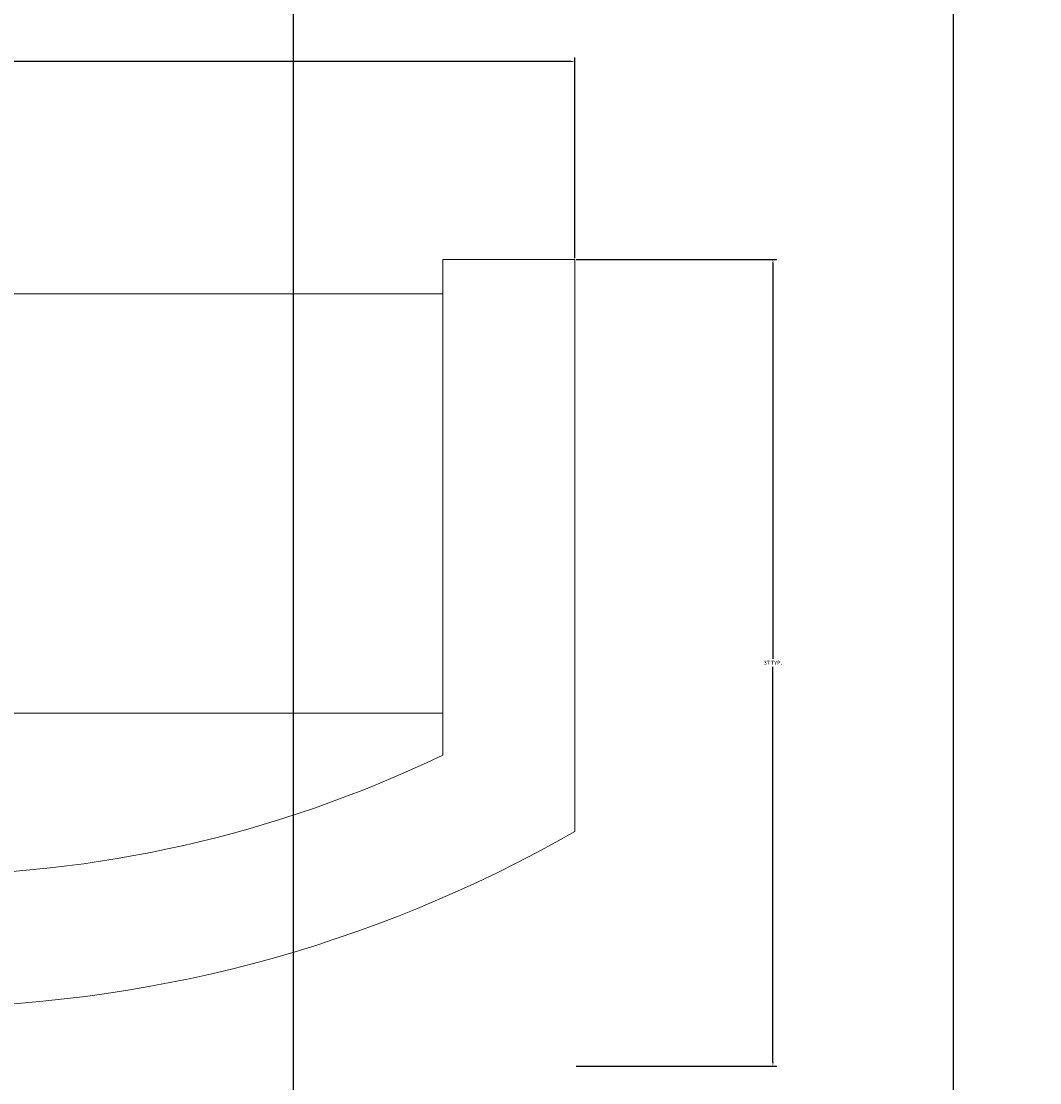
# Model space of a CAD drawing. Units: inches. Extents: x 7359 to 7979, y 33027 to 34263.
# Tile 24 of 32: x 7550 to 7597, y 33777 to 33825. Entities that reach past the tile are written whole.
import ezdxf

# ---------------------------------------------------------------- set-up
doc = ezdxf.new("R2010")
doc.units = ezdxf.units.IN
doc.layers.add('A-ANNO-DIMS', color=2, linetype='Continuous', lineweight=18)
doc.layers.add('A-FURN', color=8, linetype='Continuous', lineweight=18)
doc.styles.get("Standard").update_dxf_attribs({"font": 'arial.ttf'})
doc.dimstyles.get("Standard").update_dxf_attribs({"dimtxt": 0.18, "dimasz": 0.18, "dimexe": 0.18, "dimexo": 0.0625, "dimgap": 0.09, "dimtad": 0, "dimtih": 1, "dimtoh": 1, "dimdec": 4, "dimzin": 0, "dimdsep": 46, "dimtxsty": 'Standard', "dimcen": 0.09, "dimadec": 0, "dimazin": 0, "dimtfac": 1, "dimtdec": 4, "dimtofl": 0, "dimtmove": 0, "dimatfit": 3, "dimfxl": 1, "dimtolj": 1, "dimtzin": 0, "dimarcsym": 0})

# ---------------------------------------------------------------- blocks, each defined once
blk = doc.blocks.new('Sofa - Roundback Loveseat 5 ft.')
for p, q in [((24.00004, -33.99998), (24.00004, -11.46958)), ((-23.9998, -13.38178), (23.99986, -13.38178)), ((-24, -32.44198), (24.00004, -32.44198))]:
    blk.add_line(p, q)
blk.add_lwpolyline([(30.00004, -7.99998), (30.00004, -33.99998), (24.00004, -33.99998)])
for centre, radius, start, end in [((0, -60.24998), 60.24998, 60.13715, 119.8628), ((0, -61.38438), 55.38444, 64.32083, 115.6792)]:
    blk.add_arc(centre, radius, start, end)
blk = doc.blocks.new('*D26')
at = {"layer": 'A-ANNO-DIMS', "color": 0, "lineweight": -2, "transparency": 16777216}
for p, q in [((7515.397, 33814.613), (7515.397, 33823.731)), ((7515.577, 33823.551), (7544.174, 33823.551)), ((7575.217, 33823.551), (7546.62, 33823.551)), ((7575.397, 33814.613), (7575.397, 33823.731))]:
    blk.add_line(p, q, dxfattribs=at)
at = {"layer": 'A-ANNO-DIMS', "color": 0, "transparency": 16777216}
for points in [[(7515.577, 33823.581), (7515.577, 33823.521), (7515.397, 33823.551)], [(7575.217, 33823.581), (7575.217, 33823.521), (7575.397, 33823.551)]]:
    blk.add_solid(points, dxfattribs=at)
at = {"layer": 'Defpoints', "color": 0, "transparency": 16777216}
for p in [(7575.397, 33823.551), (7515.397, 33814.551), (7575.397, 33814.551)]:
    blk.add_point(p, dxfattribs=at)
at = {"layer": 'A-ANNO-DIMS', "color": 0, "transparency": 16777216, "insert": (7545.397, 33823.551), "char_height": 0.18, "attachment_point": 5}
blk.add_mtext('\\A1;LOVESEAT 60 TYP.', dxfattribs=at)
blk = doc.blocks.new('*D27')
at = {"layer": 'A-ANNO-DIMS', "color": 0, "lineweight": -2, "transparency": 16777216}
for p, q in [((7575.459, 33814.551), (7584.577, 33814.551)), ((7584.397, 33814.371), (7584.397, 33796.4)), ((7584.397, 33778.064), (7584.397, 33796.036)), ((7575.459, 33777.884), (7584.577, 33777.884))]:
    blk.add_line(p, q, dxfattribs=at)
at = {"layer": 'A-ANNO-DIMS', "color": 0, "transparency": 16777216}
for points in [[(7584.367, 33814.371), (7584.427, 33814.371), (7584.397, 33814.551)], [(7584.367, 33778.064), (7584.427, 33778.064), (7584.397, 33777.884)]]:
    blk.add_solid(points, dxfattribs=at)
at = {"layer": 'Defpoints', "color": 0, "transparency": 16777216}
for p in [(7575.397, 33814.551), (7575.397, 33777.884), (7584.397, 33777.884)]:
    blk.add_point(p, dxfattribs=at)
at = {"layer": 'A-ANNO-DIMS', "color": 0, "transparency": 16777216, "insert": (7584.397, 33796.218), "char_height": 0.18, "attachment_point": 5}
blk.add_mtext('\\A1;37 TYP.', dxfattribs=at)
blk = doc.blocks.new('*D68')
at = {"layer": 'A-ANNO-DIMS', "color": 0, "lineweight": -2, "transparency": 16777216}
for p, q in [((7562.591, 34181.771), (7562.591, 33632.309)), ((7592.591, 34181.771), (7592.591, 33632.309)), ((7562.771, 33632.489), (7577.373, 33632.489)), ((7592.411, 33632.489), (7577.81, 33632.489))]:
    blk.add_line(p, q, dxfattribs=at)
at = {"layer": 'A-ANNO-DIMS', "color": 0, "transparency": 16777216}
for points in [[(7562.771, 33632.519), (7562.771, 33632.459), (7562.591, 33632.489)], [(7592.411, 33632.519), (7592.411, 33632.459), (7592.591, 33632.489)]]:
    blk.add_solid(points, dxfattribs=at)
at = {"layer": 'Defpoints', "color": 0, "transparency": 16777216}
for p in [(7562.591, 34181.834), (7592.591, 34181.834), (7592.591, 33632.489)]:
    blk.add_point(p, dxfattribs=at)
at = {"layer": 'A-ANNO-DIMS', "color": 0, "transparency": 16777216, "insert": (7577.591, 33632.489), "char_height": 0.18, "attachment_point": 5}
blk.add_mtext('\\A1;30', dxfattribs=at)
blk = doc.blocks.new('*D83')
at = {"layer": 'A-ANNO-DIMS', "color": 0, "lineweight": -2, "transparency": 16777216}
for p, q in [((7592.591484, 34081.771428), (7592.591484, 33632.309146)), ((7598.591484, 34081.771428), (7598.591484, 33632.309146)), ((7592.771484, 33632.489146), (7595.442057, 33632.489146)), ((7598.411484, 33632.489146), (7595.740911, 33632.489146))]:
    blk.add_line(p, q, dxfattribs=at)
at = {"layer": 'A-ANNO-DIMS', "color": 0, "transparency": 16777216}
for points in [[(7592.771484, 33632.519146), (7592.771484, 33632.459146), (7592.591484, 33632.489146)], [(7598.411484, 33632.519146), (7598.411484, 33632.459146), (7598.591484, 33632.489146)]]:
    blk.add_solid(points, dxfattribs=at)
at = {"layer": 'Defpoints', "color": 0, "transparency": 16777216}
for p in [(7592.591484, 34081.833928), (7598.591484, 34081.833928), (7598.591484, 33632.489146)]:
    blk.add_point(p, dxfattribs=at)
at = {"layer": 'A-ANNO-DIMS', "color": 0, "transparency": 16777216, "insert": (7595.591484, 33632.489146), "char_height": 0.18, "attachment_point": 5}
blk.add_mtext('\\A1;6', dxfattribs=at)

msp = doc.modelspace()

# ---------------------------------------------------------------- block references
at = {"layer": 'A-FURN', "xscale": -1, "rotation": 180}
msp.add_blockref('Sofa - Roundback Loveseat 5 ft.', (7545.3969, 33780.551), dxfattribs=at)

# ---------------------------------------------------------------- dimensions: what is measured, and where the dimension line sits
at = {"layer": 'A-ANNO-DIMS'}
for base, p1, p2, picture, middle in [((7592.5915, 33632.4891), (7562.5915, 34181.8339), (7592.5915, 34181.8339), '*D68', (7577.5915, 33632.4891)), ((7598.5915, 33632.4891), (7592.5915, 34081.8339), (7598.5915, 34081.8339), '*D83', (7595.5915, 33632.4891))]:
    dim = msp.add_linear_dim(base=base, p1=p1, p2=p2, dimstyle='Standard', override={"dimdec": 0, "dimlfac": 1, "dimrnd": 0, "dimzin": 0, "dimdsep": 46, "dimlunit": 2}, dxfattribs=at)
    dim.commit()
    dim.dimension.update_dxf_attribs({"geometry": picture, "text_midpoint": middle})
dim = msp.add_linear_dim(base=(7575.397, 33823.551), p1=(7515.3969, 33814.551), p2=(7575.397, 33814.551), text='LOVESEAT <> TYP.', dimstyle='Standard', override={"dimdec": 0, "dimlfac": 1, "dimrnd": 0, "dimzin": 0, "dimdsep": 46, "dimlunit": 2}, dxfattribs=at)
dim.commit()
dim.dimension.update_dxf_attribs({"geometry": '*D26', "text_midpoint": (7545.397, 33823.551)})
dim = msp.add_linear_dim(base=(7584.397, 33777.8843), p1=(7575.397, 33814.551), p2=(7575.397, 33777.8843), angle=270, text='<> TYP.', dimstyle='Standard', override={"dimdec": 0, "dimlfac": 1, "dimrnd": 0, "dimzin": 0, "dimdsep": 46, "dimlunit": 2}, dxfattribs=at)
dim.commit()
dim.dimension.update_dxf_attribs({"geometry": '*D27', "text_midpoint": (7584.397, 33796.2176)})

doc.saveas('drawing.dxf')
